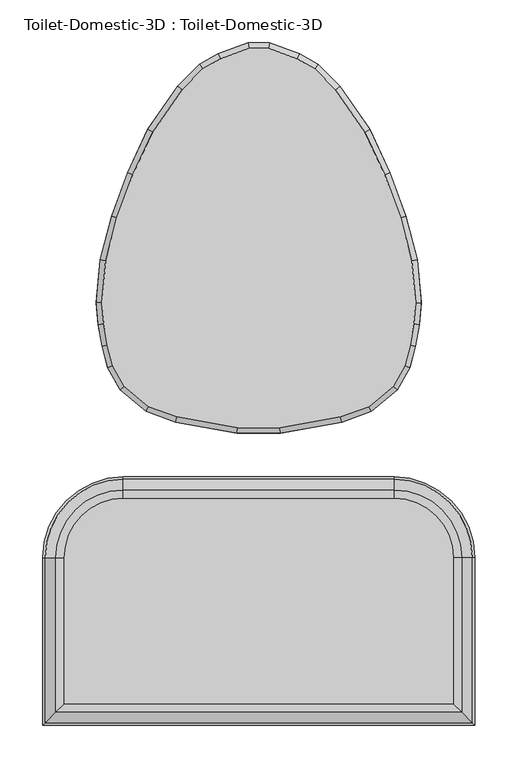
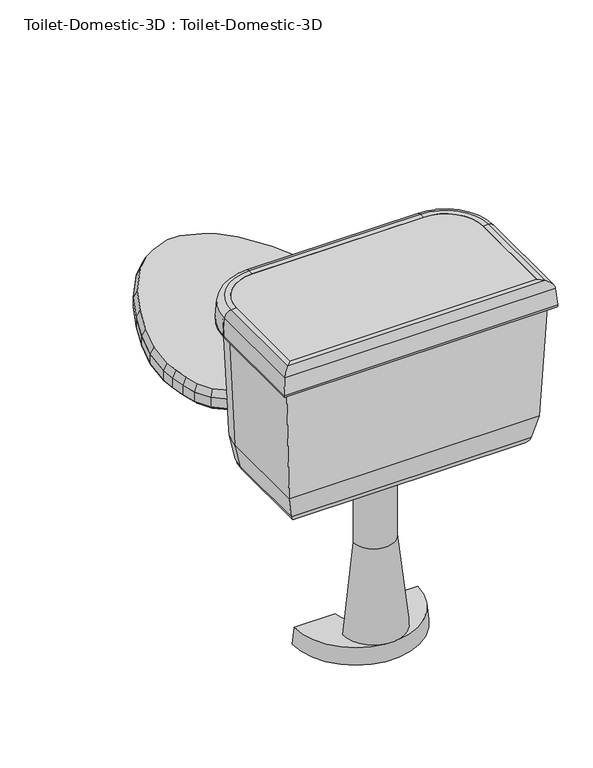
"""IFC4 building model written with IfcOpenShell, lengths in millimetres: flow terminal geometry, Toilet-Domestic-3D : Toilet-Domestic-3D."""

from ifc_helpers import new_model, si_unit, point, frame, frame_2d, origin, place, context, project, spatial, polyline, circle_curve, ellipse_curve, trimmed, segment, composite_curve, outline, extrude, faceted_brep, source, transform, mapped, element, save
from ifc_brep_helpers import plane_surface, cylinder_surface, revolved_surface, advanced_brep


def toilet_domestic_3d_toilet_domestic_3d_e67c3c64(model_context):
    return source(origin(), model_context, "Body", "SolidModel", [
        advanced_brep(
        [(177.8, -419.1, 387.2181453), (177.8, -298.45, 387.2181453), (177.8, -298.45, 374.65), (177.8, -419.1, 374.65), (192.8020829, -434.1020829, 387.2181453), (192.8020829, -298.45, 387.2181453), (211.4650931, -452.7650931, 402.4478636), (211.4650931, -298.45, 402.4478636), (218.7732506, -460.0732506, 438.15), (218.7732506, -298.45, 438.15), (228.5868869, -469.8868869, 654.05), (228.5868869, -298.45, 654.05), (228.5868869, -469.8868869, 704.85), (228.5868869, -298.45, 704.85), (237.91817, -479.21817, 704.85), (237.91817, -298.45, 704.85), (250.5698426, -491.8698426, 693.2568779), (250.5698426, -298.45, 693.2568779), (253.3960274, -494.6960274, 660.953439), (253.3960274, -298.45, 660.953439), (247.070191, -488.370191, 654.05), (247.070191, -298.45, 654.05), (241.3, -482.6, 654.05), (241.3, -298.45, 654.05), (231.4863636, -472.7863636, 438.15), (231.4863636, -298.45, 438.15), (222.3416824, -463.6416824, 393.4759963), (222.3416824, -298.45, 393.4759963), (197.8071664, -439.1071664, 374.65), (197.8071664, -298.45, 374.65), (158.75, -279.4, 387.2181453), (158.75, -279.4, 374.65), (158.75, -264.3979171, 387.2181453), (158.75, -245.7349069, 402.4478636), (158.75, -238.4267494, 438.15), (158.75, -228.6131131, 654.05), (158.75, -228.6131131, 704.85), (158.75, -219.28183, 704.85), (158.75, -206.6301574, 693.2568779), (158.75, -203.8039726, 660.953439), (158.75, -210.129809, 654.05), (158.75, -215.9, 654.05), (158.75, -225.7136364, 438.15), (158.75, -234.8583176, 393.4759963), (158.75, -259.3928336, 374.65), (-158.75, -279.4, 387.2181453), (-158.75, -279.4, 374.65), (-158.75, -264.3979171, 387.2181453), (-158.75, -245.7349069, 402.4478636), (-158.75, -238.4267494, 438.15), (-158.75, -228.6131131, 654.05), (-158.75, -228.6131131, 704.85), (-158.75, -219.28183, 704.85), (-158.75, -206.6301574, 693.2568779), (-158.75, -203.8039726, 660.953439), (-158.75, -210.129809, 654.05), (-158.75, -215.9, 654.05), (-158.75, -225.7136364, 438.15), (-158.75, -234.8583176, 393.4759963), (-158.75, -259.3928336, 374.65), (-177.8, -298.45, 387.2181453), (-177.8, -298.45, 374.65), (-192.8020829, -298.45, 387.2181453), (-211.4650931, -298.45, 402.4478636), (-218.7732506, -298.45, 438.15), (-228.5868869, -298.45, 654.05), (-228.5868869, -298.45, 704.85), (-237.91817, -298.45, 704.85), (-250.5698426, -298.45, 693.2568779), (-253.3960274, -298.45, 660.953439), (-247.070191, -298.45, 654.05), (-241.3, -298.45, 654.05), (-231.4863636, -298.45, 438.15), (-222.3416824, -298.45, 393.4759963), (-197.8071664, -298.45, 374.65), (-177.8, -419.1, 387.2181453), (-177.8, -419.1, 374.65), (-192.8020829, -434.1020829, 387.2181453), (-211.4650931, -452.7650931, 402.4478636), (-218.7732506, -460.0732506, 438.15), (-228.5868869, -469.8868869, 654.05), (-228.5868869, -469.8868869, 704.85), (-237.91817, -479.21817, 704.85), (-250.5698426, -491.8698426, 693.2568779), (-253.3960274, -494.6960274, 660.953439), (-247.070191, -488.370191, 654.05), (-241.3, -482.6, 654.05), (-231.4863636, -472.7863636, 438.15), (-222.3416824, -463.6416824, 393.4759963), (-197.8071664, -439.1071664, 374.65)],
        [
            (0, 1),
            (1, 2),
            (2, 3),
            (3, 0),
            (4, 5),
            (5, 1),
            (0, 4),
            (6, 7),
            (7, 5, circle_curve(frame((192.8020829, -298.45, 406.2681453), z_axis=(0.0, 1.0, 0.0), x_axis=(1.0, 0.0, 0.0)), 19.05)),
            (4, 6, ellipse_curve(frame((192.8020829, -434.1020829, 406.2681453), z_axis=(-0.7071067811865451, -0.7071067811865498, 0.0), x_axis=(-0.7071067811865497, 0.7071067811865452, 0.0)), 26.9407684, 19.05)),
            (8, 9),
            (9, 7),
            (6, 8),
            (10, 11),
            (11, 9),
            (8, 10),
            (12, 13),
            (13, 11),
            (10, 12),
            (14, 15),
            (15, 13),
            (12, 14),
            (16, 17),
            (17, 15, circle_curve(frame((237.91817, -298.45, 692.15), z_axis=(0.0, -1.0, 0.0), x_axis=(1.0, 0.0, 0.0)), 12.7)),
            (14, 16, ellipse_curve(frame((237.91817, -479.21817, 692.15), z_axis=(0.7071067811865451, 0.7071067811865498, 0.0), x_axis=(0.7071067811865497, -0.7071067811865452, 0.0)), 17.9605122, 12.7)),
            (18, 19),
            (19, 17),
            (16, 18),
            (20, 21),
            (21, 19, circle_curve(frame((247.070191, -298.45, 660.4), z_axis=(0.0, -1.0, 0.0), x_axis=(1.0, 0.0, 0.0)), 6.35)),
            (18, 20, ellipse_curve(frame((247.070191, -488.370191, 660.4), z_axis=(0.7071067811865451, 0.7071067811865498, 0.0), x_axis=(0.7071067811865497, -0.7071067811865452, 0.0)), 8.9802561, 6.35)),
            (22, 23),
            (23, 21),
            (20, 22),
            (24, 25),
            (25, 23),
            (22, 24),
            (26, 27),
            (27, 25),
            (24, 26),
            (28, 29),
            (29, 27, circle_curve(frame((197.8071664, -298.45, 400.05), z_axis=(0.0, -1.0, 0.0), x_axis=(1.0, 0.0, 0.0)), 25.4)),
            (26, 28, ellipse_curve(frame((197.8071664, -439.1071664, 400.05), z_axis=(0.7071067811865451, 0.7071067811865498, 0.0), x_axis=(0.7071067811865497, -0.7071067811865452, 0.0)), 35.9210245, 25.4)),
            (2, 29),
            (28, 3),
            (30, 31),
            (31, 2, circle_curve(frame((158.75, -298.45, 374.65), z_axis=(0.0, 0.0, -1.0), x_axis=(1.0, 0.0, 0.0)), 19.05)),
            (1, 30, circle_curve(frame((158.75, -298.45, 387.2181453), z_axis=(0.0, 0.0, 1.0), x_axis=(1.0, 0.0, 0.0)), 19.05)),
            (32, 30),
            (5, 32, circle_curve(frame((158.75, -298.45, 387.2181453), z_axis=(0.0, 0.0, 1.0), x_axis=(1.0, 0.0, 0.0)), 34.0520829)),
            (33, 32, circle_curve(frame((158.75, -264.3979171, 406.2681453), z_axis=(-1.0, 0.0, 0.0), x_axis=(0.0, 1.0, 0.0)), 19.05)),
            (7, 33, circle_curve(frame((158.75, -298.45, 402.4478636), z_axis=(0.0, 0.0, 1.0), x_axis=(1.0, 0.0, 0.0)), 52.7150931)),
            (34, 33),
            (9, 34, circle_curve(frame((158.75, -298.45, 438.15), z_axis=(0.0, 0.0, 1.0), x_axis=(1.0, 0.0, 0.0)), 60.0232506)),
            (35, 34),
            (11, 35, circle_curve(frame((158.75, -298.45, 654.05), z_axis=(0.0, 0.0, 1.0), x_axis=(1.0, 0.0, 0.0)), 69.8368869)),
            (36, 35),
            (13, 36, circle_curve(frame((158.75, -298.45, 704.85), z_axis=(0.0, 0.0, 1.0), x_axis=(1.0, 0.0, 0.0)), 69.8368869)),
            (37, 36),
            (15, 37, circle_curve(frame((158.75, -298.45, 704.85), z_axis=(0.0, 0.0, 1.0), x_axis=(1.0, 0.0, 0.0)), 79.16817)),
            (38, 37, circle_curve(frame((158.75, -219.28183, 692.15), z_axis=(1.0, 0.0, 0.0), x_axis=(0.0, 1.0, 0.0)), 12.7)),
            (17, 38, circle_curve(frame((158.75, -298.45, 693.2568779), z_axis=(0.0, 0.0, 1.0), x_axis=(1.0, 0.0, 0.0)), 91.8198426)),
            (39, 38),
            (19, 39, circle_curve(frame((158.75, -298.45, 660.953439), z_axis=(0.0, 0.0, 1.0), x_axis=(1.0, 0.0, 0.0)), 94.6460274)),
            (40, 39, circle_curve(frame((158.75, -210.129809, 660.4), z_axis=(1.0, 0.0, 0.0), x_axis=(0.0, 1.0, 0.0)), 6.35)),
            (21, 40, circle_curve(frame((158.75, -298.45, 654.05), z_axis=(0.0, 0.0, 1.0), x_axis=(1.0, 0.0, 0.0)), 88.320191)),
            (41, 40),
            (23, 41, circle_curve(frame((158.75, -298.45, 654.05), z_axis=(0.0, 0.0, 1.0), x_axis=(1.0, 0.0, 0.0)), 82.55)),
            (42, 41),
            (25, 42, circle_curve(frame((158.75, -298.45, 438.15), z_axis=(0.0, 0.0, 1.0), x_axis=(1.0, 0.0, 0.0)), 72.7363636)),
            (43, 42),
            (27, 43, circle_curve(frame((158.75, -298.45, 393.4759963), z_axis=(0.0, 0.0, 1.0), x_axis=(1.0, 0.0, 0.0)), 63.5916824)),
            (44, 43, circle_curve(frame((158.75, -259.3928336, 400.05), z_axis=(1.0, 0.0, 0.0), x_axis=(0.0, 1.0, 0.0)), 25.4)),
            (29, 44, circle_curve(frame((158.75, -298.45, 374.65), z_axis=(0.0, 0.0, 1.0), x_axis=(1.0, 0.0, 0.0)), 39.0571664)),
            (31, 44),
            (30, 45),
            (45, 46),
            (46, 31),
            (32, 47),
            (47, 45),
            (33, 48),
            (48, 47, circle_curve(frame((-158.75, -264.3979171, 406.2681453), z_axis=(-1.0, 0.0, 0.0), x_axis=(0.0, 1.0, 0.0)), 19.05)),
            (34, 49),
            (49, 48),
            (35, 50),
            (50, 49),
            (36, 51),
            (51, 50),
            (37, 52),
            (52, 51),
            (38, 53),
            (53, 52, circle_curve(frame((-158.75, -219.28183, 692.15), z_axis=(1.0, 0.0, 0.0), x_axis=(0.0, 1.0, 0.0)), 12.7)),
            (39, 54),
            (54, 53),
            (40, 55),
            (55, 54, circle_curve(frame((-158.75, -210.129809, 660.4), z_axis=(1.0, 0.0, 0.0), x_axis=(0.0, 1.0, 0.0)), 6.35)),
            (41, 56),
            (56, 55),
            (42, 57),
            (57, 56),
            (43, 58),
            (58, 57),
            (44, 59),
            (59, 58, circle_curve(frame((-158.75, -259.3928336, 400.05), z_axis=(1.0, 0.0, 0.0), x_axis=(0.0, 1.0, 0.0)), 25.4)),
            (46, 59),
            (60, 61),
            (61, 46, circle_curve(frame((-158.75, -298.45, 374.65), z_axis=(0.0, 0.0, -1.0), x_axis=(0.0, 1.0, 0.0)), 19.05)),
            (45, 60, circle_curve(frame((-158.75, -298.45, 387.2181453), z_axis=(0.0, 0.0, 1.0), x_axis=(0.0, 1.0, 0.0)), 19.05)),
            (62, 60),
            (47, 62, circle_curve(frame((-158.75, -298.45, 387.2181453), z_axis=(0.0, 0.0, 1.0), x_axis=(0.0, 1.0, 0.0)), 34.0520829)),
            (63, 62, circle_curve(frame((-192.8020829, -298.45, 406.2681453), z_axis=(0.0, -1.0, 0.0), x_axis=(-1.0, 0.0, 0.0)), 19.05)),
            (48, 63, circle_curve(frame((-158.75, -298.45, 402.4478636), z_axis=(0.0, 0.0, 1.0), x_axis=(0.0, 1.0, 0.0)), 52.7150931)),
            (64, 63),
            (49, 64, circle_curve(frame((-158.75, -298.45, 438.15), z_axis=(0.0, 0.0, 1.0), x_axis=(0.0, 1.0, 0.0)), 60.0232506)),
            (65, 64),
            (50, 65, circle_curve(frame((-158.75, -298.45, 654.05), z_axis=(0.0, 0.0, 1.0), x_axis=(0.0, 1.0, 0.0)), 69.8368869)),
            (66, 65),
            (51, 66, circle_curve(frame((-158.75, -298.45, 704.85), z_axis=(0.0, 0.0, 1.0), x_axis=(0.0, 1.0, 0.0)), 69.8368869)),
            (67, 66),
            (52, 67, circle_curve(frame((-158.75, -298.45, 704.85), z_axis=(0.0, 0.0, 1.0), x_axis=(0.0, 1.0, 0.0)), 79.16817)),
            (68, 67, circle_curve(frame((-237.91817, -298.45, 692.15), z_axis=(0.0, 1.0, 0.0), x_axis=(-1.0, 0.0, 0.0)), 12.7)),
            (53, 68, circle_curve(frame((-158.75, -298.45, 693.2568779), z_axis=(0.0, 0.0, 1.0), x_axis=(0.0, 1.0, 0.0)), 91.8198426)),
            (69, 68),
            (54, 69, circle_curve(frame((-158.75, -298.45, 660.953439), z_axis=(0.0, 0.0, 1.0), x_axis=(0.0, 1.0, 0.0)), 94.6460274)),
            (70, 69, circle_curve(frame((-247.070191, -298.45, 660.4), z_axis=(0.0, 1.0, 0.0), x_axis=(-1.0, 0.0, 0.0)), 6.35)),
            (55, 70, circle_curve(frame((-158.75, -298.45, 654.05), z_axis=(0.0, 0.0, 1.0), x_axis=(0.0, 1.0, 0.0)), 88.320191)),
            (71, 70),
            (56, 71, circle_curve(frame((-158.75, -298.45, 654.05), z_axis=(0.0, 0.0, 1.0), x_axis=(0.0, 1.0, 0.0)), 82.55)),
            (72, 71),
            (57, 72, circle_curve(frame((-158.75, -298.45, 438.15), z_axis=(0.0, 0.0, 1.0), x_axis=(0.0, 1.0, 0.0)), 72.7363636)),
            (73, 72),
            (58, 73, circle_curve(frame((-158.75, -298.45, 393.4759963), z_axis=(0.0, 0.0, 1.0), x_axis=(0.0, 1.0, 0.0)), 63.5916824)),
            (74, 73, circle_curve(frame((-197.8071664, -298.45, 400.05), z_axis=(0.0, 1.0, 0.0), x_axis=(-1.0, 0.0, 0.0)), 25.4)),
            (59, 74, circle_curve(frame((-158.75, -298.45, 374.65), z_axis=(0.0, 0.0, 1.0), x_axis=(0.0, 1.0, 0.0)), 39.0571664)),
            (61, 74),
            (60, 75),
            (75, 76),
            (76, 61),
            (62, 77),
            (77, 75),
            (63, 78),
            (78, 77, ellipse_curve(frame((-192.8020829, -434.1020829, 406.2681453), z_axis=(0.7071067811865498, -0.7071067811865451, 0.0), x_axis=(-0.7071067811865451, -0.70710678118655, 0.0)), 26.9407684, 19.05)),
            (64, 79),
            (79, 78),
            (65, 80),
            (80, 79),
            (66, 81),
            (81, 80),
            (67, 82),
            (82, 81),
            (68, 83),
            (83, 82, ellipse_curve(frame((-237.91817, -479.21817, 692.15), z_axis=(-0.7071067811865498, 0.7071067811865451, 0.0), x_axis=(0.7071067811865451, 0.70710678118655, 0.0)), 17.9605122, 12.7)),
            (69, 84),
            (84, 83),
            (70, 85),
            (85, 84, ellipse_curve(frame((-247.070191, -488.370191, 660.4), z_axis=(-0.7071067811865498, 0.7071067811865451, 0.0), x_axis=(0.7071067811865451, 0.70710678118655, 0.0)), 8.9802561, 6.35)),
            (71, 86),
            (86, 85),
            (72, 87),
            (87, 86),
            (73, 88),
            (88, 87),
            (74, 89),
            (89, 88, ellipse_curve(frame((-197.8071664, -439.1071664, 400.05), z_axis=(-0.7071067811865498, 0.7071067811865451, 0.0), x_axis=(0.7071067811865451, 0.70710678118655, 0.0)), 35.9210245, 25.4)),
            (76, 89),
            (75, 0),
            (3, 76),
            (77, 4),
            (78, 6),
            (79, 8),
            (80, 10),
            (81, 12),
            (82, 14),
            (83, 16),
            (84, 18),
            (85, 20),
            (86, 22),
            (87, 24),
            (88, 26),
            (89, 28),
        ],
        [
            plane_surface(frame((177.8, -419.1, 374.65), z_axis=(-1.0, 0.0, 0.0), x_axis=(0.0, 1.0, 0.0))),
            plane_surface(frame((177.8, -419.1, 387.2181453), z_axis=(0.0, 0.0, 1.0), x_axis=(0.0, 1.0, 0.0))),
            revolved_surface(polyline([(211.8520829, -298.45, 406.2681453), (211.8520829, -453.1520829260162, 406.2681453)]), (192.8020829, -419.1, 406.2681453), (0.0, 1.0, 0.0)),
            plane_surface(frame((211.4650931, -452.7650931, 402.4478636), z_axis=(-0.9796855721787505, 0.0, 0.2005397209153197), x_axis=(0.0, 1.0, 0.0))),
            plane_surface(frame((218.7732506, -460.0732506, 438.15), z_axis=(-0.9989685402102995, 0.0, 0.045407660918654086), x_axis=(0.0, 1.0, 0.0))),
            plane_surface(frame((228.5868869, -469.8868869, 654.05), z_axis=(-1.0, 0.0, 0.0), x_axis=(0.0, 1.0, 0.0))),
            plane_surface(frame((228.5868869, -469.8868869, 704.85), z_axis=(0.0, 0.0, 1.0), x_axis=(0.0, 1.0, 0.0))),
            cylinder_surface(frame((237.91817, -419.1, 692.15), z_axis=(0.0, -1.0, 0.0), x_axis=(1.0, 0.0, 0.0)), 12.7),
            plane_surface(frame((250.5698426, -491.8698426, 693.2568779), z_axis=(0.9961946980917452, 0.0, 0.08715574274766269), x_axis=(0.0, 1.0, 0.0))),
            cylinder_surface(frame((247.070191, -419.1, 660.4), z_axis=(0.0, -1.0, 0.0), x_axis=(1.0, 0.0, 0.0)), 6.35),
            plane_surface(frame((247.070191, -488.370191, 654.05), z_axis=(0.0, 0.0, -1.0), x_axis=(0.0, 1.0, 0.0))),
            plane_surface(frame((241.3, -482.6, 654.05), z_axis=(0.9989685402102993, 0.0, -0.04540766091865594), x_axis=(0.0, 1.0, 0.0))),
            plane_surface(frame((231.4863636, -472.7863636, 438.15), z_axis=(0.9796855721787489, 0.0, -0.20053972091532798), x_axis=(0.0, 1.0, 0.0))),
            cylinder_surface(frame((197.8071664, -419.1, 400.05), z_axis=(0.0, -1.0, 0.0), x_axis=(1.0, 0.0, 0.0)), 25.4),
            plane_surface(frame((197.8071664, -439.1071664, 374.65), z_axis=(0.0, 0.0, -1.0), x_axis=(0.0, 1.0, 0.0))),
            revolved_surface(polyline([(177.8, -298.45, 374.65), (177.8, -298.45, 387.2181453)]), (158.75, -298.45, 0.0), (0.0, 0.0, -1.0)),
            plane_surface(frame((158.75, -298.45, 387.2181453), z_axis=(0.0, 0.0, 1.0), x_axis=(1.0, 0.0, 0.0))),
            revolved_surface(trimmed(ellipse_curve(frame((192.8020829, -298.45, 406.2681453), z_axis=(0.0, -1.0, 0.0), x_axis=(1.0, 0.0, 0.0)), 19.05, 19.05), [point((192.8020829, -298.45, 387.2181453))], [point((211.4650931, -298.45, 402.4478636))], True, "CARTESIAN"), (158.75, -298.45, 0.0), (0.0, 0.0, -1.0)),
            revolved_surface(polyline([(211.4650931, -298.45, 402.4478636), (218.7732506, -298.45, 438.15)]), (158.75, -298.45, 0.0), (0.0, 0.0, -1.0)),
            revolved_surface(polyline([(218.7732506, -298.45, 438.15), (228.5868869, -298.45, 654.05)]), (158.75, -298.45, 0.0), (0.0, 0.0, -1.0)),
            revolved_surface(polyline([(228.5868869, -298.45, 654.05), (228.5868869, -298.45, 704.85)]), (158.75, -298.45, 0.0), (0.0, 0.0, -1.0)),
            plane_surface(frame((158.75, -298.45, 704.85), z_axis=(0.0, 0.0, 1.0), x_axis=(1.0, 0.0, 0.0))),
            revolved_surface(trimmed(ellipse_curve(frame((237.91817, -298.45, 692.15), z_axis=(0.0, 1.0, 0.0), x_axis=(1.0, 0.0, 0.0)), 12.7, 12.7), [point((237.91817, -298.45, 704.85))], [point((250.5698426, -298.45, 693.2568779))], True, "CARTESIAN"), (158.75, -298.45, 0.0), (0.0, 0.0, -1.0)),
            revolved_surface(polyline([(250.5698426, -298.45, 693.2568779), (253.3960274, -298.45, 660.953439)]), (158.75, -298.45, 0.0), (0.0, 0.0, -1.0)),
            revolved_surface(trimmed(ellipse_curve(frame((247.070191, -298.45, 660.4), z_axis=(0.0, 1.0, 0.0), x_axis=(1.0, 0.0, 0.0)), 6.35, 6.35), [point((253.3960274, -298.45, 660.953439))], [point((247.070191, -298.45, 654.05))], True, "CARTESIAN"), (158.75, -298.45, 0.0), (0.0, 0.0, -1.0)),
            plane_surface(frame((158.75, -298.45, 654.05), z_axis=(0.0, 0.0, -1.0), x_axis=(1.0, 0.0, 0.0))),
            revolved_surface(polyline([(241.3, -298.45, 654.05), (231.4863636, -298.45, 438.15)]), (158.75, -298.45, 0.0), (0.0, 0.0, -1.0)),
            revolved_surface(polyline([(231.4863636, -298.45, 438.15), (222.3416824, -298.45, 393.4759963)]), (158.75, -298.45, 0.0), (0.0, 0.0, -1.0)),
            revolved_surface(trimmed(ellipse_curve(frame((197.8071664, -298.45, 400.05), z_axis=(0.0, 1.0, 0.0), x_axis=(1.0, 0.0, 0.0)), 25.4, 25.4), [point((222.3416824, -298.45, 393.4759963))], [point((197.8071664, -298.45, 374.65))], True, "CARTESIAN"), (158.75, -298.45, 0.0), (0.0, 0.0, -1.0)),
            plane_surface(frame((158.75, -298.45, 374.65), z_axis=(0.0, 0.0, -1.0), x_axis=(1.0, 0.0, 0.0))),
            plane_surface(frame((158.75, -279.4, 374.65), z_axis=(0.0, -1.0, 0.0), x_axis=(-1.0, 0.0, 0.0))),
            plane_surface(frame((158.75, -279.4, 387.2181453), z_axis=(0.0, 0.0, 1.0), x_axis=(-1.0, 0.0, 0.0))),
            revolved_surface(polyline([(-158.75, -245.34791709999996, 406.2681453), (158.75, -245.34791709999996, 406.2681453)]), (158.75, -264.3979171, 406.2681453), (-1.0, 0.0, 0.0)),
            plane_surface(frame((158.75, -245.7349069, 402.4478636), z_axis=(0.0, -0.9796855721787505, 0.2005397209153197), x_axis=(-1.0, 0.0, 0.0))),
            plane_surface(frame((158.75, -238.4267494, 438.15), z_axis=(0.0, -0.9989685402102995, 0.045407660918654086), x_axis=(-1.0, 0.0, 0.0))),
            plane_surface(frame((158.75, -228.6131131, 654.05), z_axis=(0.0, -1.0, 0.0), x_axis=(-1.0, 0.0, 0.0))),
            plane_surface(frame((158.75, -228.6131131, 704.85), z_axis=(0.0, 0.0, 1.0), x_axis=(-1.0, 0.0, 0.0))),
            cylinder_surface(frame((158.75, -219.28183, 692.15), z_axis=(1.0, 0.0, 0.0), x_axis=(0.0, 1.0, 0.0)), 12.7),
            plane_surface(frame((158.75, -206.6301574, 693.2568779), z_axis=(0.0, 0.9961946980917452, 0.08715574274766269), x_axis=(-1.0, 0.0, 0.0))),
            cylinder_surface(frame((158.75, -210.129809, 660.4), z_axis=(1.0, 0.0, 0.0), x_axis=(0.0, 1.0, 0.0)), 6.35),
            plane_surface(frame((158.75, -210.129809, 654.05), z_axis=(0.0, 0.0, -1.0), x_axis=(-1.0, 0.0, 0.0))),
            plane_surface(frame((158.75, -215.9, 654.05), z_axis=(0.0, 0.9989685402102993, -0.04540766091865594), x_axis=(-1.0, 0.0, 0.0))),
            plane_surface(frame((158.75, -225.7136364, 438.15), z_axis=(0.0, 0.9796855721787489, -0.20053972091532798), x_axis=(-1.0, 0.0, 0.0))),
            cylinder_surface(frame((158.75, -259.3928336, 400.05), z_axis=(1.0, 0.0, 0.0), x_axis=(0.0, 1.0, 0.0)), 25.4),
            plane_surface(frame((158.75, -259.3928336, 374.65), z_axis=(0.0, 0.0, -1.0), x_axis=(-1.0, 0.0, 0.0))),
            revolved_surface(polyline([(-158.75, -279.4, 374.65), (-158.75, -279.4, 387.2181453)]), (-158.75, -298.45, 0.0), (0.0, 0.0, -1.0)),
            plane_surface(frame((-158.75, -298.45, 387.2181453), z_axis=(0.0, 0.0, 1.0), x_axis=(0.0, 1.0, 0.0))),
            revolved_surface(trimmed(ellipse_curve(frame((-158.75, -264.3979171, 406.2681453), z_axis=(1.0, 0.0, 0.0), x_axis=(0.0, 1.0, 0.0)), 19.05, 19.05), [point((-158.75, -264.3979171, 387.2181453))], [point((-158.75, -245.7349069, 402.4478636))], True, "CARTESIAN"), (-158.75, -298.45, 0.0), (0.0, 0.0, -1.0)),
            revolved_surface(polyline([(-158.75, -245.7349069, 402.4478636), (-158.75, -238.4267494, 438.15)]), (-158.75, -298.45, 0.0), (0.0, 0.0, -1.0)),
            revolved_surface(polyline([(-158.75, -238.4267494, 438.15), (-158.75, -228.6131131, 654.05)]), (-158.75, -298.45, 0.0), (0.0, 0.0, -1.0)),
            revolved_surface(polyline([(-158.75, -228.6131131, 654.05), (-158.75, -228.6131131, 704.85)]), (-158.75, -298.45, 0.0), (0.0, 0.0, -1.0)),
            plane_surface(frame((-158.75, -298.45, 704.85), z_axis=(0.0, 0.0, 1.0), x_axis=(0.0, 1.0, 0.0))),
            revolved_surface(trimmed(ellipse_curve(frame((-158.75, -219.28183, 692.15), z_axis=(-1.0, 0.0, 0.0), x_axis=(0.0, 1.0, 0.0)), 12.7, 12.7), [point((-158.75, -219.28183, 704.85))], [point((-158.75, -206.6301574, 693.2568779))], True, "CARTESIAN"), (-158.75, -298.45, 0.0), (0.0, 0.0, -1.0)),
            revolved_surface(polyline([(-158.75, -206.6301574, 693.2568779), (-158.75, -203.8039726, 660.953439)]), (-158.75, -298.45, 0.0), (0.0, 0.0, -1.0)),
            revolved_surface(trimmed(ellipse_curve(frame((-158.75, -210.129809, 660.4), z_axis=(-1.0, 0.0, 0.0), x_axis=(0.0, 1.0, 0.0)), 6.35, 6.35), [point((-158.75, -203.8039726, 660.953439))], [point((-158.75, -210.129809, 654.05))], True, "CARTESIAN"), (-158.75, -298.45, 0.0), (0.0, 0.0, -1.0)),
            plane_surface(frame((-158.75, -298.45, 654.05), z_axis=(0.0, 0.0, -1.0), x_axis=(0.0, 1.0, 0.0))),
            revolved_surface(polyline([(-158.75, -215.9, 654.05), (-158.75, -225.7136364, 438.15)]), (-158.75, -298.45, 0.0), (0.0, 0.0, -1.0)),
            revolved_surface(polyline([(-158.75, -225.7136364, 438.15), (-158.75, -234.8583176, 393.4759963)]), (-158.75, -298.45, 0.0), (0.0, 0.0, -1.0)),
            revolved_surface(trimmed(ellipse_curve(frame((-158.75, -259.3928336, 400.05), z_axis=(-1.0, 0.0, 0.0), x_axis=(0.0, 1.0, 0.0)), 25.4, 25.4), [point((-158.75, -234.8583176, 393.4759963))], [point((-158.75, -259.3928336, 374.65))], True, "CARTESIAN"), (-158.75, -298.45, 0.0), (0.0, 0.0, -1.0)),
            plane_surface(frame((-158.75, -298.45, 374.65), z_axis=(0.0, 0.0, -1.0), x_axis=(0.0, 1.0, 0.0))),
            plane_surface(frame((-177.8, -298.45, 374.65), z_axis=(1.0, 0.0, 0.0), x_axis=(0.0, -1.0, 0.0))),
            plane_surface(frame((-177.8, -298.45, 387.2181453), z_axis=(0.0, 0.0, 1.0), x_axis=(0.0, -1.0, 0.0))),
            revolved_surface(polyline([(-211.8520829, -453.15208292601636, 406.2681453), (-211.8520829, -298.45, 406.2681453)]), (-192.8020829, -298.45, 406.2681453), (0.0, -1.0, 0.0)),
            plane_surface(frame((-211.4650931, -298.45, 402.4478636), z_axis=(0.9796855721787505, 0.0, 0.2005397209153197), x_axis=(0.0, -1.0, 0.0))),
            plane_surface(frame((-218.7732506, -298.45, 438.15), z_axis=(0.9989685402102995, 0.0, 0.045407660918654086), x_axis=(0.0, -1.0, 0.0))),
            plane_surface(frame((-228.5868869, -298.45, 654.05), z_axis=(1.0, 0.0, 0.0), x_axis=(0.0, -1.0, 0.0))),
            plane_surface(frame((-228.5868869, -298.45, 704.85), z_axis=(0.0, 0.0, 1.0), x_axis=(0.0, -1.0, 0.0))),
            cylinder_surface(frame((-237.91817, -298.45, 692.15), z_axis=(0.0, 1.0, 0.0), x_axis=(-1.0, 0.0, 0.0)), 12.7),
            plane_surface(frame((-250.5698426, -298.45, 693.2568779), z_axis=(-0.9961946980917452, 0.0, 0.08715574274766269), x_axis=(0.0, -1.0, 0.0))),
            cylinder_surface(frame((-247.070191, -298.45, 660.4), z_axis=(0.0, 1.0, 0.0), x_axis=(-1.0, 0.0, 0.0)), 6.35),
            plane_surface(frame((-247.070191, -298.45, 654.05), z_axis=(0.0, 0.0, -1.0), x_axis=(0.0, -1.0, 0.0))),
            plane_surface(frame((-241.3, -298.45, 654.05), z_axis=(-0.9989685402102993, 0.0, -0.04540766091865594), x_axis=(0.0, -1.0, 0.0))),
            plane_surface(frame((-231.4863636, -298.45, 438.15), z_axis=(-0.9796855721787489, 0.0, -0.20053972091532798), x_axis=(0.0, -1.0, 0.0))),
            cylinder_surface(frame((-197.8071664, -298.45, 400.05), z_axis=(0.0, 1.0, 0.0), x_axis=(-1.0, 0.0, 0.0)), 25.4),
            plane_surface(frame((-197.8071664, -298.45, 374.65), z_axis=(0.0, 0.0, -1.0), x_axis=(0.0, -1.0, 0.0))),
            plane_surface(frame((-177.8, -419.1, 374.65), z_axis=(0.0, 1.0, 0.0), x_axis=(1.0, 0.0, 0.0))),
            plane_surface(frame((-177.8, -419.1, 387.2181453), z_axis=(0.0, 0.0, 1.0), x_axis=(1.0, 0.0, 0.0))),
            revolved_surface(polyline([(211.85208292601635, -453.15208290000004, 406.2681453), (-211.85208292601618, -453.15208290000004, 406.2681453)]), (-177.8, -434.1020829, 406.2681453), (1.0, 0.0, 0.0)),
            plane_surface(frame((-211.4650931, -452.7650931, 402.4478636), z_axis=(0.0, 0.9796855721787505, 0.2005397209153197), x_axis=(1.0, 0.0, 0.0))),
            plane_surface(frame((-218.7732506, -460.0732506, 438.15), z_axis=(0.0, 0.9989685402102995, 0.045407660918654086), x_axis=(1.0, 0.0, 0.0))),
            plane_surface(frame((-228.5868869, -469.8868869, 654.05), z_axis=(0.0, 1.0, 0.0), x_axis=(1.0, 0.0, 0.0))),
            plane_surface(frame((-228.5868869, -469.8868869, 704.85), z_axis=(0.0, 0.0, 1.0), x_axis=(1.0, 0.0, 0.0))),
            cylinder_surface(frame((-177.8, -479.21817, 692.15), z_axis=(-1.0, 0.0, 0.0), x_axis=(0.0, -1.0, 0.0)), 12.7),
            plane_surface(frame((-250.5698426, -491.8698426, 693.2568779), z_axis=(0.0, -0.9961946980917452, 0.08715574274766269), x_axis=(1.0, 0.0, 0.0))),
            cylinder_surface(frame((-177.8, -488.370191, 660.4), z_axis=(-1.0, 0.0, 0.0), x_axis=(0.0, -1.0, 0.0)), 6.35),
            plane_surface(frame((-247.070191, -488.370191, 654.05), z_axis=(0.0, 0.0, -1.0), x_axis=(1.0, 0.0, 0.0))),
            plane_surface(frame((-241.3, -482.6, 654.05), z_axis=(0.0, -0.9989685402102993, -0.04540766091865594), x_axis=(1.0, 0.0, 0.0))),
            plane_surface(frame((-231.4863636, -472.7863636, 438.15), z_axis=(0.0, -0.9796855721787489, -0.20053972091532798), x_axis=(1.0, 0.0, 0.0))),
            cylinder_surface(frame((-177.8, -439.1071664, 400.05), z_axis=(-1.0, 0.0, 0.0), x_axis=(0.0, -1.0, 0.0)), 25.4),
            plane_surface(frame((-197.8071664, -439.1071664, 374.65), z_axis=(0.0, 0.0, -1.0), x_axis=(1.0, 0.0, 0.0))),
        ],
        [
            (0, [[1, 2, 3, 4]]),
            (1, [[5, 6, -1, 7]]),
            (2, [[8, 9, -5, 10]]),
            (3, [[11, 12, -8, 13]]),
            (4, [[14, 15, -11, 16]]),
            (5, [[17, 18, -14, 19]]),
            (6, [[20, 21, -17, 22]]),
            (7, [[23, 24, -20, 25]]),
            (8, [[26, 27, -23, 28]]),
            (9, [[29, 30, -26, 31]]),
            (10, [[32, 33, -29, 34]]),
            (11, [[35, 36, -32, 37]]),
            (12, [[38, 39, -35, 40]]),
            (13, [[41, 42, -38, 43]]),
            (14, [[-3, 44, -41, 45]]),
            (15, [[46, 47, -2, 48]]),
            (16, [[49, -48, -6, 50]]),
            (17, [[51, -50, -9, 52]]),
            (18, [[53, -52, -12, 54]]),
            (19, [[55, -54, -15, 56]]),
            (20, [[57, -56, -18, 58]]),
            (21, [[59, -58, -21, 60]]),
            (22, [[61, -60, -24, 62]]),
            (23, [[63, -62, -27, 64]]),
            (24, [[65, -64, -30, 66]]),
            (25, [[67, -66, -33, 68]]),
            (26, [[69, -68, -36, 70]]),
            (27, [[71, -70, -39, 72]]),
            (28, [[73, -72, -42, 74]]),
            (29, [[75, -74, -44, -47]]),
            (30, [[76, 77, 78, -46]]),
            (31, [[79, 80, -76, -49]]),
            (32, [[81, 82, -79, -51]]),
            (33, [[83, 84, -81, -53]]),
            (34, [[85, 86, -83, -55]]),
            (35, [[87, 88, -85, -57]]),
            (36, [[89, 90, -87, -59]]),
            (37, [[91, 92, -89, -61]]),
            (38, [[93, 94, -91, -63]]),
            (39, [[95, 96, -93, -65]]),
            (40, [[97, 98, -95, -67]]),
            (41, [[99, 100, -97, -69]]),
            (42, [[101, 102, -99, -71]]),
            (43, [[103, 104, -101, -73]]),
            (44, [[-78, 105, -103, -75]]),
            (45, [[106, 107, -77, 108]]),
            (46, [[109, -108, -80, 110]]),
            (47, [[111, -110, -82, 112]]),
            (48, [[113, -112, -84, 114]]),
            (49, [[115, -114, -86, 116]]),
            (50, [[117, -116, -88, 118]]),
            (51, [[119, -118, -90, 120]]),
            (52, [[121, -120, -92, 122]]),
            (53, [[123, -122, -94, 124]]),
            (54, [[125, -124, -96, 126]]),
            (55, [[127, -126, -98, 128]]),
            (56, [[129, -128, -100, 130]]),
            (57, [[131, -130, -102, 132]]),
            (58, [[133, -132, -104, 134]]),
            (59, [[135, -134, -105, -107]]),
            (60, [[136, 137, 138, -106]]),
            (61, [[139, 140, -136, -109]]),
            (62, [[141, 142, -139, -111]]),
            (63, [[143, 144, -141, -113]]),
            (64, [[145, 146, -143, -115]]),
            (65, [[147, 148, -145, -117]]),
            (66, [[149, 150, -147, -119]]),
            (67, [[151, 152, -149, -121]]),
            (68, [[153, 154, -151, -123]]),
            (69, [[155, 156, -153, -125]]),
            (70, [[157, 158, -155, -127]]),
            (71, [[159, 160, -157, -129]]),
            (72, [[161, 162, -159, -131]]),
            (73, [[163, 164, -161, -133]]),
            (74, [[-138, 165, -163, -135]]),
            (75, [[166, -4, 167, -137]]),
            (76, [[168, -7, -166, -140]]),
            (77, [[169, -10, -168, -142]]),
            (78, [[170, -13, -169, -144]]),
            (79, [[171, -16, -170, -146]]),
            (80, [[172, -19, -171, -148]]),
            (81, [[173, -22, -172, -150]]),
            (82, [[174, -25, -173, -152]]),
            (83, [[175, -28, -174, -154]]),
            (84, [[176, -31, -175, -156]]),
            (85, [[177, -34, -176, -158]]),
            (86, [[178, -37, -177, -160]]),
            (87, [[179, -40, -178, -162]]),
            (88, [[180, -43, -179, -164]]),
            (89, [[-167, -45, -180, -165]]),
        ],
    ),
        extrude(outline(composite_curve([segment(polyline([(-38.1, -342.9), (38.1, -342.9)]), True, "CONTINUOUS"), segment(trimmed(circle_curve(frame_2d((0.0, -342.9)), 38.1), [point((38.1, -342.9))], [point((-38.1, -342.9))], False, "CARTESIAN"), True, "CONTINUOUS")], self_intersect=False)), frame((0.0, 0.0, 206.375), z_axis=(0.0, 0.0, 1.0), x_axis=(1.0, 0.0, 0.0)), (0.0, 0.0, 1.0), 130.175),
        extrude(outline(composite_curve([segment(polyline([(228.5868869, -469.8868869), (-228.5868869, -469.8868869), (-228.5868869, -298.45)]), True, "CONTINUOUS"), segment(trimmed(circle_curve(frame_2d((-158.75, -298.45)), 69.8368869), [point((-228.5868869, -298.45))], [point((-158.75, -228.6131131))], False, "CARTESIAN"), True, "CONTINUOUS"), segment(polyline([(-158.75, -228.6131131), (158.75, -228.6131131)]), True, "CONTINUOUS"), segment(trimmed(circle_curve(frame_2d((158.75, -298.45)), 69.8368869), [point((158.75, -228.6131131))], [point((228.5868869, -298.45))], False, "CARTESIAN"), True, "CONTINUOUS"), segment(polyline([(228.5868869, -298.45), (228.5868869, -469.8868869)]), True, "CONTINUOUS")], self_intersect=False)), frame((0.0, 0.0, 654.05), z_axis=(0.0, 0.0, 1.0), x_axis=(1.0, 0.0, 0.0)), (0.0, 0.0, 1.0), 50.8),
        faceted_brep([(-157.6293435, -97.472128, 400.05), (-129.0942628, -121.4159037, 400.05), (-95.7755003, -133.5429415, 400.05), (-24.844447, -146.05, 400.05), (24.844447, -146.05, 400.05), (95.7755003, -133.5429415, 400.05), (129.0942628, -121.4159037, 400.05), (157.6293435, -97.472128, 400.05), (171.060664, -73.773864, 400.05), (177.5851102, -49.4242991, 400.05), (181.9845715, -24.4737144, 400.05), (184.125744, 0.0, 400.05), (179.7950716, 49.4998127, 400.05), (166.347, 99.688699, 400.05), (148.0469602, 149.9676451, 400.05), (124.7045808, 200.0255393, 400.05), (90.0971582, 249.9125941, 400.05), (65.691017, 274.3187354, 400.05), (44.8990862, 286.3229622, 400.05), (11.5803237, 298.45, 400.05), (-11.5803237, 298.45, 400.05), (-44.8990862, 286.3229622, 400.05), (-65.691017, 274.3187354, 400.05), (-90.0971582, 249.9125941, 400.05), (-124.7045808, 200.0255393, 400.05), (-148.0469602, 149.9676451, 400.05), (-166.347, 99.688699, 400.05), (-179.7950716, 49.4998127, 400.05), (-184.125744, 0.0, 400.05), (-181.9845715, -24.4737144, 400.05), (-177.5851102, -49.4242991, 400.05), (-171.060664, -73.773864, 400.05), (-162.5887836, -101.6, 387.2181453), (-176.9845865, -76.2, 387.2181453), (-183.790496, -50.8, 387.2181453), (-188.2862441, -25.3033453, 387.2181453), (-190.5, 0.0, 387.2181453), (-186.0724883, 50.6066907, 387.2181453), (-172.4088722, 101.6, 387.2181453), (-153.9191843, 152.4, 387.2181453), (-130.2307553, 203.2, 387.2181453), (-94.9900085, 254.0, 387.2181453), (-69.5900085, 279.4, 387.2181453), (-47.5929632, 292.1, 387.2181453), (-12.7, 304.8, 387.2181453), (12.7, 304.8, 387.2181453), (47.5929632, 292.1, 387.2181453), (69.5900085, 279.4, 387.2181453), (94.9900085, 254.0, 387.2181453), (130.2307553, 203.2, 387.2181453), (153.9191843, 152.4, 387.2181453), (172.4088722, 101.6, 387.2181453), (186.0724883, 50.6066907, 387.2181453), (190.5, 0.0, 387.2181453), (188.2862441, -25.3033453, 387.2181453), (183.790496, -50.8, 387.2181453), (176.9845865, -76.2, 387.2181453), (162.5887836, -101.6, 387.2181453), (132.3182423, -127.0, 387.2181453), (97.4252791, -139.7, 387.2181453), (25.4, -152.4, 387.2181453), (-25.4, -152.4, 387.2181453), (-97.4252791, -139.7, 387.2181453), (-132.3182423, -127.0, 387.2181453)], [[[0, 1, 2, 3, 4, 5, 6, 7, 8, 9, 10, 11, 12, 13, 14, 15, 16, 17, 18, 19, 20, 21, 22, 23, 24, 25, 26, 27, 28, 29, 30, 31]], [[32, 33, 34, 35, 36, 37, 38, 39, 40, 41, 42, 43, 44, 45, 46, 47, 48, 49, 50, 51, 52, 53, 54, 55, 56, 57, 58, 59, 60, 61, 62, 63]], [[32, 0, 31, 33]], [[33, 31, 30, 34]], [[34, 30, 29, 35]], [[35, 29, 28, 36]], [[36, 28, 27, 37]], [[37, 27, 26, 38]], [[38, 26, 25, 39]], [[39, 25, 24, 40]], [[40, 24, 23, 41]], [[41, 23, 22, 42]], [[42, 22, 21, 43]], [[43, 21, 20, 44]], [[44, 20, 19, 45]], [[45, 19, 18, 46]], [[46, 18, 17, 47]], [[47, 17, 16, 48]], [[48, 16, 15, 49]], [[49, 15, 14, 50]], [[50, 14, 13, 51]], [[51, 13, 12, 52]], [[52, 12, 11, 53]], [[53, 11, 10, 54]], [[54, 10, 9, 55]], [[55, 9, 8, 56]], [[56, 8, 7, 57]], [[57, 7, 6, 58]], [[58, 6, 5, 59]], [[59, 5, 4, 60]], [[60, 4, 3, 61]], [[61, 3, 2, 62]], [[62, 2, 1, 63]], [[63, 1, 0, 32]]]),
        advanced_brep(
        [(-38.1, -342.9, 206.375), (-38.1, -342.9, 31.75), (-57.15, -342.9, 31.75), (38.1, -342.9, 206.375), (57.15, -342.9, 31.75), (38.1, -342.9, 31.75)],
        [
            (0, 1),
            (1, 2),
            (2, 0),
            (3, 4),
            (4, 5),
            (5, 3),
            (3, 0, circle_curve(frame((0.0, -342.9, 206.375), z_axis=(0.0, 0.0, -1.0), x_axis=(-1.0, 0.0, 0.0)), 38.1)),
            (2, 4, circle_curve(frame((0.0, -342.9, 31.75), z_axis=(0.0, 0.0, 1.0), x_axis=(-1.0, 0.0, 0.0)), 57.15)),
            (1, 5, circle_curve(frame((0.0, -342.9, 31.75), z_axis=(0.0, 0.0, 1.0), x_axis=(-1.0, 0.0, 0.0)), 38.1)),
        ],
        [
            plane_surface(frame((0.0, -342.9, 31.75), z_axis=(0.0, 1.0, 0.0), x_axis=(-1.0, 0.0, 0.0))),
            plane_surface(frame((0.0, -342.9, 31.75), z_axis=(0.0, 1.0, 0.0), x_axis=(1.0, 0.0, 0.0))),
            revolved_surface(polyline([(-38.1, -342.9, 206.375), (-57.15, -342.9, 31.75)]), (0.0, -342.9, 31.75), (0.0, 0.0, -1.0)),
            plane_surface(frame((0.0, -342.9, 31.75), z_axis=(0.0, 0.0, -1.0), x_axis=(-1.0, 0.0, 0.0))),
            revolved_surface(polyline([(-38.1, -342.9, 31.75), (-38.1, -342.9, 206.375)]), (0.0, -342.9, 31.75), (0.0, 0.0, -1.0)),
        ],
        [
            (0, [[1, 2, 3]]),
            (1, [[4, 5, 6]]),
            (2, [[-4, 7, -3, 8]]),
            (3, [[-5, -8, -2, 9]]),
            (4, [[-6, -9, -1, -7]]),
        ],
    ),
        advanced_brep(
        [(-117.7636364, -285.75, 0.0), (-114.3, -285.75, 31.75), (-38.1, -285.75, 31.75), (-38.1, -285.75, 0.0), (117.7636364, -285.75, 0.0), (38.1, -285.75, 0.0), (38.1, -285.75, 31.75), (114.3, -285.75, 31.75)],
        [
            (0, 1),
            (1, 2),
            (2, 3),
            (3, 0),
            (4, 5),
            (5, 6),
            (6, 7),
            (7, 4),
            (4, 0, circle_curve(frame((0.0, -285.75, 0.0), z_axis=(0.0, 0.0, -1.0), x_axis=(-1.0, 0.0, 0.0)), 117.7636364)),
            (3, 5, circle_curve(frame((0.0, -285.75, 0.0), z_axis=(0.0, 0.0, 1.0), x_axis=(-1.0, 0.0, 0.0)), 38.1)),
            (2, 6, circle_curve(frame((0.0, -285.75, 31.75), z_axis=(0.0, 0.0, 1.0), x_axis=(-1.0, 0.0, 0.0)), 38.1)),
            (1, 7, circle_curve(frame((0.0, -285.75, 31.75), z_axis=(0.0, 0.0, 1.0), x_axis=(-1.0, 0.0, 0.0)), 114.3)),
        ],
        [
            plane_surface(frame((0.0, -285.75, -304.8), z_axis=(0.0, 1.0, 0.0), x_axis=(-1.0, 0.0, 0.0))),
            plane_surface(frame((0.0, -285.75, -304.8), z_axis=(0.0, 1.0, 0.0), x_axis=(1.0, 0.0, 0.0))),
            plane_surface(frame((0.0, -285.75, 0.0), z_axis=(0.0, 0.0, -1.0), x_axis=(-1.0, 0.0, 0.0))),
            revolved_surface(polyline([(-38.1, -285.75, 0.0), (-38.1, -285.75, 31.75)]), (0.0, -285.75, -304.8), (0.0, 0.0, -1.0)),
            plane_surface(frame((0.0, -285.75, 31.75), z_axis=(0.0, 0.0, 1.0), x_axis=(-1.0, 0.0, 0.0))),
            revolved_surface(polyline([(-114.3, -285.75, 31.75), (-117.7636364, -285.75, 0.0)]), (0.0, -285.75, -304.8), (0.0, 0.0, -1.0)),
        ],
        [
            (0, [[1, 2, 3, 4]]),
            (1, [[5, 6, 7, 8]]),
            (2, [[-5, 9, -4, 10]]),
            (3, [[-6, -10, -3, 11]]),
            (4, [[-7, -11, -2, 12]]),
            (5, [[-8, -12, -1, -9]]),
        ],
    ),
        extrude(outline(composite_curve([segment(polyline([(177.8, -419.1), (-177.8, -419.1), (-177.8, -298.45)]), True, "CONTINUOUS"), segment(trimmed(circle_curve(frame_2d((-158.75, -298.45)), 19.05), [point((-177.8, -298.45))], [point((-158.75, -279.4))], False, "CARTESIAN"), True, "CONTINUOUS"), segment(polyline([(-158.75, -279.4), (158.75, -279.4)]), True, "CONTINUOUS"), segment(trimmed(circle_curve(frame_2d((158.75, -298.45)), 19.05), [point((158.75, -279.4))], [point((177.8, -298.45))], False, "CARTESIAN"), True, "CONTINUOUS"), segment(polyline([(177.8, -298.45), (177.8, -419.1)]), True, "CONTINUOUS")], self_intersect=False)), frame((0.0, 0.0, 374.65), z_axis=(0.0, 0.0, 1.0), x_axis=(1.0, 0.0, 0.0)), (0.0, 0.0, 1.0), 12.5681453),
        faceted_brep([(-97.4252791, -139.7, 368.3), (-25.4, -152.4, 368.3), (25.4, -152.4, 368.3), (97.4252791, -139.7, 368.3), (132.3182423, -127.0, 368.3), (162.5887836, -101.6, 368.3), (176.9845865, -76.2, 368.3), (183.790496, -50.8, 368.3), (188.2862441, -25.3033453, 368.3), (190.5, 0.0, 368.3), (186.0724883, 50.6066907, 368.3), (172.4088722, 101.6, 368.3), (153.9191843, 152.4, 368.3), (130.2307553, 203.2, 368.3), (94.9900085, 254.0, 368.3), (69.5900085, 279.4, 368.3), (47.5929632, 292.1, 368.3), (12.7, 304.8, 368.3), (-12.7, 304.8, 368.3), (-47.5929632, 292.1, 368.3), (-69.5900085, 279.4, 368.3), (-94.9900085, 254.0, 368.3), (-130.2307553, 203.2, 368.3), (-153.9191843, 152.4, 368.3), (-172.4088722, 101.6, 368.3), (-186.0724883, 50.6066907, 368.3), (-190.5, 0.0, 368.3), (-188.2862441, -25.3033453, 368.3), (-183.790496, -50.8, 368.3), (-176.9845865, -76.2, 368.3), (-162.5887836, -101.6, 368.3), (-132.3182423, -127.0, 368.3), (-95.7755003, -133.5429415, 361.95), (-129.0942628, -121.4159037, 361.95), (-157.6293435, -97.472128, 361.95), (-171.060664, -73.773864, 361.95), (-177.5851102, -49.4242991, 361.95), (-181.9845715, -24.4737144, 361.95), (-184.125744, 0.0, 361.95), (-179.7950716, 49.4998127, 361.95), (-166.347, 99.688699, 361.95), (-148.0469602, 149.9676451, 361.95), (-124.7045808, 200.0255393, 361.95), (-90.0971582, 249.9125941, 361.95), (-65.691017, 274.3187354, 361.95), (-44.8990862, 286.3229622, 361.95), (-11.5803237, 298.45, 361.95), (11.5803237, 298.45, 361.95), (44.8990862, 286.3229622, 361.95), (65.691017, 274.3187354, 361.95), (90.0971582, 249.9125941, 361.95), (124.7045808, 200.0255393, 361.95), (148.0469602, 149.9676451, 361.95), (166.347, 99.688699, 361.95), (179.7950716, 49.4998127, 361.95), (184.125744, 0.0, 361.95), (181.9845715, -24.4737144, 361.95), (177.5851102, -49.4242991, 361.95), (171.060664, -73.773864, 361.95), (157.6293435, -97.472128, 361.95), (129.0942628, -121.4159037, 361.95), (95.7755003, -133.5429415, 361.95), (24.844447, -146.05, 361.95), (-24.844447, -146.05, 361.95)], [[[0, 1, 2, 3, 4, 5, 6, 7, 8, 9, 10, 11, 12, 13, 14, 15, 16, 17, 18, 19, 20, 21, 22, 23, 24, 25, 26, 27, 28, 29, 30, 31]], [[32, 33, 34, 35, 36, 37, 38, 39, 40, 41, 42, 43, 44, 45, 46, 47, 48, 49, 50, 51, 52, 53, 54, 55, 56, 57, 58, 59, 60, 61, 62, 63]], [[32, 0, 31, 33]], [[33, 31, 30, 34]], [[34, 30, 29, 35]], [[35, 29, 28, 36]], [[36, 28, 27, 37]], [[37, 27, 26, 38]], [[38, 26, 25, 39]], [[39, 25, 24, 40]], [[40, 24, 23, 41]], [[41, 23, 22, 42]], [[42, 22, 21, 43]], [[43, 21, 20, 44]], [[44, 20, 19, 45]], [[45, 19, 18, 46]], [[46, 18, 17, 47]], [[47, 17, 16, 48]], [[48, 16, 15, 49]], [[49, 15, 14, 50]], [[50, 14, 13, 51]], [[51, 13, 12, 52]], [[52, 12, 11, 53]], [[53, 11, 10, 54]], [[54, 10, 9, 55]], [[55, 9, 8, 56]], [[56, 8, 7, 57]], [[57, 7, 6, 58]], [[58, 6, 5, 59]], [[59, 5, 4, 60]], [[60, 4, 3, 61]], [[61, 3, 2, 62]], [[62, 2, 1, 63]], [[63, 1, 0, 32]]]),
        extrude(outline(polyline([(-162.5887836, -101.6), (-176.9845865, -76.2), (-183.790496, -50.8), (-188.2862441, -25.3033453), (-190.5, 0.0), (-186.0724883, 50.6066907), (-172.4088722, 101.6), (-153.9191843, 152.4), (-130.2307553, 203.2), (-94.9900085, 254.0), (-69.5900085, 279.4), (-47.5929632, 292.1), (-12.7, 304.8), (12.7, 304.8), (47.5929632, 292.1), (69.5900085, 279.4), (94.9900085, 254.0), (130.2307553, 203.2), (153.9191843, 152.4), (172.4088722, 101.6), (186.0724883, 50.6066907), (190.5, 0.0), (188.2862441, -25.3033453), (183.790496, -50.8), (176.9845865, -76.2), (162.5887836, -101.6), (132.3182423, -127.0), (97.4252791, -139.7), (25.4, -152.4), (-25.4, -152.4), (-97.4252791, -139.7), (-132.3182423, -127.0), (-162.5887836, -101.6)])), frame((0.0, 0.0, 368.3), z_axis=(0.0, 0.0, 1.0), x_axis=(1.0, 0.0, 0.0)), (0.0, 0.0, 1.0), 19.05),
    ])


if __name__ == "__main__":
    model = new_model("IFC4")
    model_context = context("Model", 3, world=origin())
    ifc_project = project(units=[si_unit("LENGTHUNIT", "METRE", prefix="MILLI")], contexts=[model_context])
    site = spatial("IfcSite", under=ifc_project)
    building = spatial("IfcBuilding", under=site)
    placement = place(None, origin())
    toilet_domestic_3d_toilet_domestic_3d_shape = toilet_domestic_3d_toilet_domestic_3d_e67c3c64(model_context)
    element("IfcFlowTerminal", 1, ObjectType="Toilet-Domestic-3D : Toilet-Domestic-3D", at=placement, inside=building, context=model_context, shape_type="MappedRepresentation", body=[
        mapped(toilet_domestic_3d_toilet_domestic_3d_shape, transform((0.0, 0.0, 0.0), x_axis=(1.0, 0.0, 0.0), y_axis=(0.0, 1.0, 0.0), z_axis=(0.0, 0.0, 1.0))),
    ])
    save(model, "model.ifc")

# Revit data of these elements
# Type "Toilet-Domestic-3D : Toilet-Domestic-3D"
#   Assembly Code = "D2010110"
#   Toilet - Bowl/Basin Material = Porcelain, Linen
#   Toilet - Seat Material = Laminate, Linen, Matte
#   Default Elevation = 0
# Element 1 (IfcFlowTerminal, "Toilet-Domestic-3D : Toilet-Domestic-3D")
#   Materials on its faces: "Porcelain, Linen", "Laminate, Linen, Matte"
# Materials
#   "Porcelain, Linen": class "Ceramic", colour RGB 249 239 230, transparency 0, Description = "Porcelain, linen", Cost = 0
#   "Laminate, Linen, Matte": class "Plastic", colour RGB 249 239 230, transparency 0, Description = "Plastic Laminate - Linen, Matte", Cost = 0
